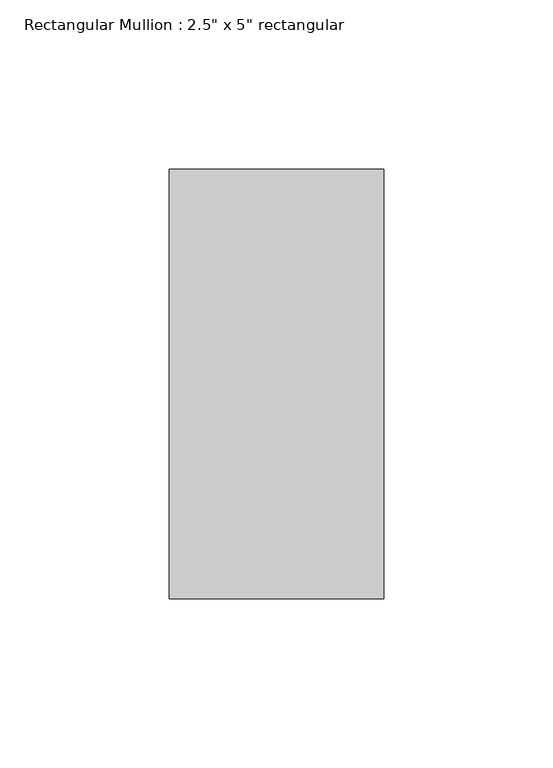
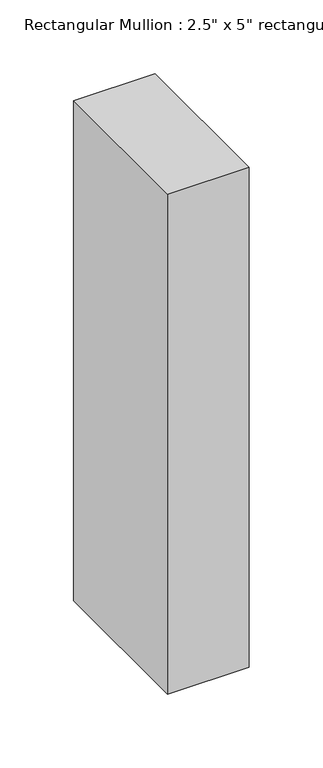
"""IFC4 building model written with IfcOpenShell, lengths in millimetres: member geometry."""

from ifc_helpers import new_model, si_unit, frame, origin, place, context, project, spatial, polyline, outline, extrude, source, transform, mapped, element, save


def member_5ae8a700(model_context):
    return source(origin(), model_context, "Body", "SweptSolid", [
        extrude(outline(polyline([(31.75, 63.5), (31.75, -63.5), (-31.75, -63.5), (-31.75, 63.5), (31.75, 63.5)])), frame((0.0, 0.0, -412.75), z_axis=(0.0, 0.0, 1.0), x_axis=(1.0, 0.0, 0.0)), (0.0, 0.0, 1.0), 412.75),
    ])


if __name__ == "__main__":
    model = new_model("IFC4")
    model_context = context("Model", 3, world=origin())
    ifc_project = project(units=[si_unit("LENGTHUNIT", "METRE", prefix="MILLI")], contexts=[model_context])
    site = spatial("IfcSite", under=ifc_project)
    building = spatial("IfcBuilding", under=site)
    placement = place(None, origin())
    member_shape = member_5ae8a700(model_context)
    element("IfcMember", 1, ObjectType="Rectangular Mullion : 2.5\" x 5\" rectangular", at=placement, inside=building, context=model_context, shape_type="MappedRepresentation", body=[
        mapped(member_shape, transform((0.0, 0.0, 0.0), x_axis=(1.0, 0.0, 0.0), y_axis=(0.0, 1.0, 0.0), z_axis=(0.0, 0.0, 1.0))),
    ])
    save(model, "model.ifc")

# Revit data of these elements
# Type "Rectangular Mullion : 2.5\" x 5\" rectangular"
#   built-in parameter 1007304 = 0.416667 (stored number, unit not read)
#   built-in parameter 1007301 = 0.104167 (stored number, unit not read)
#   built-in parameter 1007300 = 0.104167 (stored number, unit not read)
# Element 1 (IfcMember, "Rectangular Mullion : 2.5\" x 5\" rectangular")
#   Materials on its faces: "door colour"
# Materials
#   "door colour": class "Generic", colour RGB 120 120 120, transparency 0, Cost = 0
